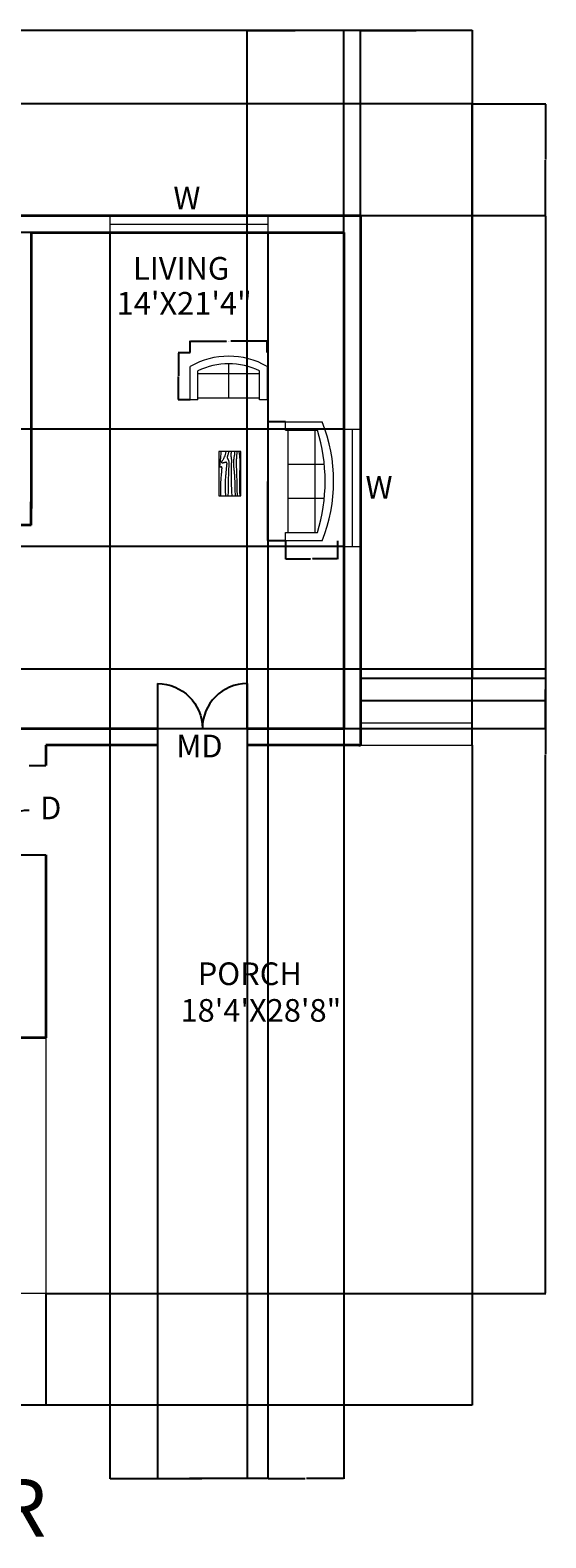
# Model space of a CAD drawing. Units: feet. Extents: x 2270 to 3094, y 1543 to 2352.
# Tile 6 of 6: x 2817 to 3094, y 1543 to 2352. Entities that reach past the tile are written whole.
import ezdxf

# ---------------------------------------------------------------- set-up
doc = ezdxf.new("R2010")
doc.units = ezdxf.units.FT
for name, color, linetype, lineweight in [('A-ANNO-DIMS', 2, 'Continuous', 18), ('A-ANNO-TEXT', 7, 'Continuous', 18), ('A-ANNO-TITL', 7, 'Continuous', 35), ('A-AREA-IDEN', 7, 'Continuous', 18), ('A-DOOR', 3, 'Continuous', 25), ('A-FLOR', 7, 'Continuous', 25), ('A-FLOR-STRS', 7, 'Continuous', 18), ('A-FURN', 8, 'Continuous', 18), ('A-GLAZ', 4, 'Continuous', 18), ('A-WALL', 7, 'Continuous', 35), ('C-PROP', 8, 'Continuous', 25)]:
    doc.layers.add(name, color=color, linetype=linetype, lineweight=lineweight)
doc.styles.get("Standard").update_dxf_attribs({"font": 'arial.ttf'})
doc.dimstyles.get("Standard").update_dxf_attribs({"dimtxt": 0.18, "dimasz": 0.18, "dimexe": 0.18, "dimexo": 0.0625, "dimgap": 0.09, "dimtad": 0, "dimtih": 1, "dimtoh": 1, "dimdec": 4, "dimzin": 0, "dimdsep": 46, "dimtxsty": 'Standard', "dimcen": 0.09, "dimadec": 0, "dimazin": 0, "dimtfac": 1, "dimtdec": 4, "dimtofl": 0, "dimtmove": 0, "dimatfit": 3, "dimfxl": 1, "dimtolj": 1, "dimtzin": 0, "dimarcsym": 0})

# ---------------------------------------------------------------- blocks, each defined once
blk = doc.blocks.new('Sofa - Roundback 7 ft.')
for p, q in [((-12.00002, -32.4421), (-12.00003, -6.5971)), ((11.99997, -32.4421), (11.99998, -6.5971)), ((-36.000027, -34), (-36.000027, -11.4696)), ((-35.999844, -13.3819), (35.9998, -13.3819)), ((35.99998, -34), (35.99998, -11.4696)), ((-36.000027, -32.4421), (35.99998, -32.4421))]:
    blk.add_line(p, q)
for points in [[(-36.000027, -34), (-42.000027, -34), (-42.000027, -8)], [(41.99998, -8), (41.99998, -34), (35.99998, -34)]]:
    blk.add_lwpolyline(points)
for centre, radius, start, end in [((0, -114.25), 114.25, 68.43141, 111.5686), ((-0.00001, -127.1968), 121.1968, 72.72033, 107.2797)]:
    blk.add_arc(centre, radius, start, end)
blk = doc.blocks.new('Sofa - Roundback Loveseat 5 ft.')
for p, q in [((-24, -33.99998), (-24, -11.46958)), ((0, -32.44198), (0, -5.99998)), ((24.00004, -33.99998), (24.00004, -11.46958)), ((-23.9998, -13.38178), (23.99986, -13.38178)), ((-24, -32.44198), (24.00004, -32.44198))]:
    blk.add_line(p, q)
for points in [[(-24, -33.99998), (-30, -33.99998), (-30, -7.99998)], [(30.00004, -7.99998), (30.00004, -33.99998), (24.00004, -33.99998)]]:
    blk.add_lwpolyline(points)
for centre, radius, start, end in [((0, -60.24998), 60.24998, 60.13715, 119.8628), ((0, -61.38438), 55.38444, 64.32083, 115.6792)]:
    blk.add_arc(centre, radius, start, end)
blk = doc.blocks.new('Table - Rectangular Woodgrain 60 x 30 in.')
for p, q in [((0, 0), (0, -30)), ((60, 0), (0, 0)), ((60, -30), (60, 0)), ((0, -30), (60, -30))]:
    blk.add_line(p, q)
for points in [[(0, -2.4), (4.8155, -2.418), (9.0302, -2.4688), (12.709, -2.5477), (15.9167, -2.65), (18.7181, -2.7711), (21.1781, -2.9063), (23.3616, -3.0508), (25.3333, -3.2), (27.1477, -3.3495), (28.8172, -3.4958), (30.3437, -3.636), (31.7291, -3.7667), (32.9756, -3.8849), (34.0849, -3.9875), (35.059, -4.0714), (35.9, -4.1334), (36.6114, -4.1711), (37.2041, -4.1854), (37.6906, -4.1779), (38.0833, -4.15), (38.3948, -4.1034), (38.6375, -4.0396), (38.8239, -3.9602), (38.9666, -3.8667), (39.0764, -3.7608), (39.1573, -3.6448), (39.2116, -3.521), (39.2416, -3.3917), (39.2498, -3.2593), (39.2385, -3.1261), (39.21, -2.9944), (39.1666, -2.8667), (39.111, -2.7447), (39.0468, -2.6281), (38.978, -2.5163), (38.9083, -2.4083), (38.8418, -2.3035), (38.7823, -2.201), (38.7337, -2.1001), (38.7, -2), (38.6844, -1.9003), (38.6875, -1.8021), (38.7094, -1.707), (38.75, -1.6167), (38.8094, -1.5326), (38.8875, -1.4563), (38.9844, -1.3893), (39.1, -1.3333), (39.2351, -1.2896), (39.3937, -1.2583), (39.5804, -1.2396), (39.8, -1.2333), (40.057, -1.2396), (40.3562, -1.2583), (40.7023, -1.2896), (41.1, -1.3333), (41.5547, -1.3895), (42.0755, -1.4573), (42.6721, -1.5361), (43.3542, -1.625), (44.1316, -1.7233), (45.014, -1.8302), (46.0114, -1.9449), (47.1333, -2.0667), (48.3862, -2.1947), (49.7625, -2.3281), (51.2513, -2.4663), (52.8416, -2.6083), (54.5226, -2.7535), (56.2833, -2.9011), (58.1127, -3.0501), (60, -3.2)], [(0, -9.2), (6.5759, -9.0858), (11.9385, -9.0365), (16.2527, -9.0418), (19.6833, -9.0917), (22.3952, -9.1759), (24.5531, -9.2844), (26.322, -9.4069), (27.8666, -9.5333), (29.3241, -9.6553), (30.7203, -9.7719), (32.0532, -9.8837), (33.3208, -9.9917), (34.5213, -10.0965), (35.6526, -10.199), (36.7128, -10.2999), (37.7, -10.4), (38.6129, -10.4996), (39.4531, -10.5969), (40.223, -10.6895), (40.925, -10.775), (41.5613, -10.8512), (42.1344, -10.9156), (42.6465, -10.966), (43.1, -11), (43.4976, -11.0158), (43.8437, -11.0136), (44.143, -10.9942), (44.4, -10.9583), (44.6195, -10.9069), (44.8062, -10.8406), (44.9648, -10.7603), (45.1, -10.6667), (45.2155, -10.5598), (45.3114, -10.4365), (45.3871, -10.2929), (45.4416, -10.125), (45.4743, -9.929), (45.4844, -9.7011), (45.4709, -9.4371), (45.4333, -9.1333), (45.3716, -8.7883), (45.2896, -8.4104), (45.1919, -8.0107), (45.0833, -7.6), (44.9685, -7.1893), (44.8521, -6.7896), (44.7388, -6.4117), (44.6333, -6.0667), (44.54, -5.7628), (44.4614, -5.4979), (44.4001, -5.2675), (44.3583, -5.0667), (44.3384, -4.8909), (44.3427, -4.7354), (44.3736, -4.5956), (44.4333, -4.4667), (44.5236, -4.3453), (44.6427, -4.2333), (44.7884, -4.1339), (44.9583, -4.05), (45.1501, -3.9849), (45.3614, -3.9417), (45.59, -3.9234), (45.8333, -3.9333), (46.0915, -3.9749), (46.3734, -4.0531), (46.6906, -4.1736), (47.0542, -4.3417), (47.4756, -4.5629), (47.9661, -4.8427), (48.5372, -5.1866), (49.2, -5.6), (49.9676, -6.0844), (50.8594, -6.625), (51.8965, -7.2031), (53.1, -7.8), (54.491, -8.3969), (56.0906, -8.975), (57.9199, -9.5156), (60, -10)], [(0, -12.8), (5.1847, -12.9322), (9.6213, -13.0323), (13.3963, -13.1059), (16.5958, -13.1583), (19.3063, -13.1952), (21.614, -13.2219), (23.6054, -13.2439), (25.3666, -13.2667), (26.9728, -13.2947), (28.4531, -13.3281), (29.8256, -13.3663), (31.1083, -13.4083), (32.3191, -13.4535), (33.476, -13.501), (34.597, -13.5501), (35.7, -13.6), (36.7984, -13.6497), (37.8875, -13.6979), (38.9578, -13.743), (40, -13.7833), (41.0047, -13.8174), (41.9625, -13.8438), (42.864, -13.8607), (43.7, -13.8667), (44.4631, -13.8604), (45.1552, -13.8417), (45.7801, -13.8104), (46.3416, -13.7667), (46.8439, -13.7104), (47.2906, -13.6417), (47.6858, -13.5604), (48.0333, -13.4667), (48.3375, -13.3608), (48.6042, -13.2448), (48.8396, -13.121), (49.05, -12.9917), (49.2417, -12.8593), (49.4208, -12.7261), (49.5937, -12.5944), (49.7667, -12.4667), (49.9452, -12.3451), (50.1323, -12.2313), (50.3303, -12.1268), (50.5416, -12.0333), (50.7686, -11.9524), (51.0135, -11.8854), (51.2788, -11.8341), (51.5666, -11.8), (51.8785, -11.7843), (52.2116, -11.7865), (52.562, -11.8059), (52.926, -11.8417), (53.2998, -11.8931), (53.6795, -11.9594), (54.0614, -12.0397), (54.4416, -12.1333), (54.8223, -12.2401), (55.2293, -12.3625), (55.6942, -12.5037), (56.2489, -12.6667), (56.9251, -12.8547), (57.7545, -13.0708), (58.7689, -13.3182), (60, -13.6)], [(0, -18), (5.124, -17.7273), (9.6609, -17.5057), (13.6705, -17.3303), (17.2125, -17.1958), (20.3467, -17.0973), (23.1328, -17.0297), (25.6307, -16.9878), (27.9, -16.9667), (29.9928, -16.9617), (31.9302, -16.9703), (33.7254, -16.9907), (35.3917, -17.0208), (36.9423, -17.0588), (38.3906, -17.1026), (39.7499, -17.1503), (41.0333, -17.2), (42.2519, -17.2496), (43.4073, -17.2969), (44.4986, -17.3395), (45.525, -17.375), (46.4858, -17.4012), (47.3802, -17.4156), (48.2074, -17.416), (48.9667, -17.4), (49.6583, -17.3662), (50.2872, -17.3167), (50.8595, -17.2547), (51.3812, -17.1833), (51.8584, -17.1057), (52.2971, -17.025), (52.7034, -16.9443), (53.0833, -16.8667), (53.443, -16.7951), (53.789, -16.7313), (54.128, -16.6768), (54.4666, -16.6334), (54.8115, -16.6024), (55.1693, -16.5854), (55.5465, -16.5841), (55.95, -16.6), (56.3828, -16.6337), (56.8346, -16.6823), (57.2915, -16.7418), (57.7396, -16.8084), (58.165, -16.878), (58.5539, -16.9469), (58.8924, -17.0111), (59.1666, -17.0667), (59.3679, -17.1107), (59.5078, -17.1438), (59.6032, -17.1675), (59.6708, -17.1833), (59.7275, -17.193), (59.7901, -17.1979), (59.8753, -17.1998), (60, -17.2)], [(0, -22.4), (8.0098, -22.2501), (14.4094, -22.1011), (19.4168, -21.9535), (23.25, -21.8083), (26.1269, -21.6663), (28.2656, -21.5281), (29.884, -21.3947), (31.2, -21.2667), (32.3967, -21.1448), (33.5172, -21.0292), (34.5697, -20.9198), (35.5625, -20.8167), (36.5037, -20.7198), (37.4015, -20.6292), (38.2642, -20.5448), (39.1, -20.4667), (39.9164, -20.3951), (40.7187, -20.3313), (41.5117, -20.2768), (42.3, -20.2333), (43.0883, -20.2024), (43.8812, -20.1854), (44.6836, -20.1841), (45.5, -20.2), (46.3328, -20.234), (47.1747, -20.2844), (48.0163, -20.3488), (48.8479, -20.425), (49.66, -20.5106), (50.4429, -20.6031), (51.1872, -20.7004), (51.8833, -20.8), (52.5246, -20.8999), (53.1166, -20.9995), (53.6681, -21.0983), (54.1875, -21.1958), (54.6834, -21.2919), (55.1646, -21.3859), (55.6394, -21.4777), (56.1167, -21.5667), (56.6028, -21.6515), (57.0961, -21.7266), (57.5929, -21.7852), (58.0896, -21.8208), (58.5823, -21.8268), (59.0674, -21.7964), (59.5412, -21.723), (60, -21.6)], [(0, -25.2), (8.6355, -25.0504), (15.7026, -24.9031), (21.4049, -24.7606), (25.9458, -24.625), (29.529, -24.4988), (32.3578, -24.3844), (34.6359, -24.284), (36.5667, -24.2), (38.3213, -24.1341), (39.9417, -24.0854), (41.437, -24.0523), (42.8167, -24.0333), (44.0901, -24.0268), (45.2667, -24.0313), (46.3557, -24.0451), (47.3667, -24.0667), (48.309, -24.0947), (49.1928, -24.1287), (50.0284, -24.168), (50.826, -24.2125), (51.5959, -24.2617), (52.3483, -24.3151), (53.0935, -24.3725), (53.8417, -24.4334), (54.6009, -24.497), (55.3699, -24.561), (56.1454, -24.6226), (56.9239, -24.6792), (57.7021, -24.7279), (58.4764, -24.7662), (59.2435, -24.7911), (60, -24.8)], [(0, -28.8), (5.6867, -28.6681), (10.45, -28.5698), (14.407, -28.5012), (17.675, -28.4584), (20.3711, -28.4374), (22.6125, -28.4344), (24.5164, -28.4455), (26.2, -28.4667), (27.762, -28.4947), (29.2276, -28.5281), (30.6033, -28.5663), (31.8958, -28.6084), (33.1118, -28.6535), (34.2578, -28.7011), (35.3405, -28.7501), (36.3666, -28.8), (37.3443, -28.8497), (38.288, -28.8974), (39.2137, -28.9412), (40.1375, -28.9792), (41.0753, -29.0093), (42.0432, -29.0297), (43.0572, -29.0384), (44.1333, -29.0333), (45.2936, -29.0114), (46.5843, -28.9641), (48.0579, -28.8816), (49.7666, -28.7542), (51.7629, -28.5721), (54.0989, -28.3255), (56.8272, -28.0048), (60, -27.6)]]:
    blk.add_lwpolyline(points)
blk = doc.blocks.new('DOOR-SWING-24')
blk.add_line((33, 0), (0, 0))
blk.add_arc((9, 0), 24, 0, 90)
blk = doc.blocks.new('*D18')
at = {"layer": 'A-ANNO-DIMS', "color": 0, "lineweight": -2, "transparency": 16777216}
for p, q in [((2954.26, 2141.51), (2944.57, 2141.51)), ((2944.75, 2141.33), (2944.75, 2109.77)), ((2944.75, 2077.85), (2944.75, 2109.41)), ((2954.26, 2077.67), (2944.57, 2077.67))]:
    blk.add_line(p, q, dxfattribs=at)
at = {"layer": 'A-ANNO-DIMS', "color": 0, "transparency": 16777216}
for points in [[(2944.72, 2141.33), (2944.78, 2141.33), (2944.75, 2141.51)], [(2944.72, 2077.85), (2944.78, 2077.85), (2944.75, 2077.67)]]:
    blk.add_solid(points, dxfattribs=at)
at = {"layer": 'Defpoints', "color": 0, "transparency": 16777216}
for p in [(2954.33, 2141.51), (2944.75, 2077.67), (2954.33, 2077.67)]:
    blk.add_point(p, dxfattribs=at)
at = {"layer": 'A-ANNO-DIMS', "color": 0, "transparency": 16777216, "insert": (2944.75, 2109.59), "char_height": 0.18, "attachment_point": 5}
blk.add_mtext('\\A1;SOFA 64 TYP.', dxfattribs=at)
blk = doc.blocks.new('*D19')
at = {"layer": 'A-ANNO-DIMS', "color": 0, "lineweight": -2, "transparency": 16777216}
for p, q in [((2954.33, 2077.6), (2954.33, 2067.91)), ((2982.2, 2077.6), (2982.2, 2067.91)), ((2954.51, 2068.09), (2967.73, 2068.09)), ((2982.02, 2068.09), (2968.79, 2068.09))]:
    blk.add_line(p, q, dxfattribs=at)
at = {"layer": 'A-ANNO-DIMS', "color": 0, "transparency": 16777216}
for points in [[(2954.51, 2068.12), (2954.51, 2068.06), (2954.33, 2068.09)], [(2982.02, 2068.12), (2982.02, 2068.06), (2982.2, 2068.09)]]:
    blk.add_solid(points, dxfattribs=at)
at = {"layer": 'Defpoints', "color": 0, "transparency": 16777216}
for p in [(2954.33, 2077.67), (2982.2, 2077.67), (2982.2, 2068.09)]:
    blk.add_point(p, dxfattribs=at)
at = {"layer": 'A-ANNO-DIMS', "color": 0, "transparency": 16777216, "insert": (2968.26, 2068.09), "char_height": 0.18, "attachment_point": 5}
blk.add_mtext('\\A1;28 TYP.', dxfattribs=at)
blk = doc.blocks.new('*D20')
at = {"layer": 'A-ANNO-DIMS', "color": 0, "lineweight": -2, "transparency": 16777216}
for p, q in [((2903.14, 2178.61), (2903.14, 2184.93)), ((2903.32, 2184.75), (2922.59, 2184.75)), ((2944.3, 2184.75), (2925.04, 2184.75)), ((2944.48, 2178.61), (2944.48, 2184.93))]:
    blk.add_line(p, q, dxfattribs=at)
at = {"layer": 'A-ANNO-DIMS', "color": 0, "transparency": 16777216}
for points in [[(2903.32, 2184.78), (2903.32, 2184.72), (2903.14, 2184.75)], [(2944.3, 2184.78), (2944.3, 2184.72), (2944.48, 2184.75)]]:
    blk.add_solid(points, dxfattribs=at)
at = {"layer": 'Defpoints', "color": 0, "transparency": 16777216}
for p in [(2944.48, 2184.75), (2903.14, 2178.55), (2944.48, 2178.55)]:
    blk.add_point(p, dxfattribs=at)
at = {"layer": 'A-ANNO-DIMS', "color": 0, "transparency": 16777216, "insert": (2923.81, 2184.75), "char_height": 0.18, "attachment_point": 5}
blk.add_mtext('\\A1;LOVESEAT 41 TYP.', dxfattribs=at)
blk = doc.blocks.new('*D21')
at = {"layer": 'A-ANNO-DIMS', "color": 0, "lineweight": -2, "transparency": 16777216}
for p, q in [((2903.08, 2178.55), (2896.76, 2178.55)), ((2896.94, 2178.37), (2896.94, 2166.1)), ((2896.94, 2153.46), (2896.94, 2165.73)), ((2903.08, 2153.28), (2896.76, 2153.28))]:
    blk.add_line(p, q, dxfattribs=at)
at = {"layer": 'A-ANNO-DIMS', "color": 0, "transparency": 16777216}
for points in [[(2896.91, 2178.37), (2896.97, 2178.37), (2896.94, 2178.55)], [(2896.91, 2153.46), (2896.97, 2153.46), (2896.94, 2153.28)]]:
    blk.add_solid(points, dxfattribs=at)
at = {"layer": 'Defpoints', "color": 0, "transparency": 16777216}
for p in [(2896.94, 2178.55), (2903.14, 2178.55), (2903.14, 2153.28)]:
    blk.add_point(p, dxfattribs=at)
at = {"layer": 'A-ANNO-DIMS', "color": 0, "transparency": 16777216, "insert": (2896.94, 2165.92), "char_height": 0.18, "attachment_point": 5}
blk.add_mtext('\\A1;25 TYP.', dxfattribs=at)
blk = doc.blocks.new('*D26')
at = {"layer": 'A-ANNO-DIMS', "color": 0, "lineweight": -2, "transparency": 16777216}
for p, q in [((2309.67, 2312.15), (2309.67, 2351.56)), ((2309.85, 2351.38), (2681.88, 2351.38)), ((3054.49, 2351.38), (2682.45, 2351.38)), ((3054.67, 2312.15), (3054.67, 2351.56))]:
    blk.add_line(p, q, dxfattribs=at)
at = {"layer": 'A-ANNO-DIMS', "color": 0, "transparency": 16777216}
for points in [[(2309.85, 2351.41), (2309.85, 2351.35), (2309.67, 2351.38)], [(3054.49, 2351.41), (3054.49, 2351.35), (3054.67, 2351.38)]]:
    blk.add_solid(points, dxfattribs=at)
at = {"layer": 'Defpoints', "color": 0, "transparency": 16777216}
for p in [(3054.67, 2351.38), (2309.67, 2312.08), (3054.67, 2312.08)]:
    blk.add_point(p, dxfattribs=at)
at = {"layer": 'A-ANNO-DIMS', "color": 0, "transparency": 16777216, "insert": (2682.17, 2351.38), "char_height": 0.18, "attachment_point": 5}
blk.add_mtext('\\A1;745', dxfattribs=at)
blk = doc.blocks.new('*D28')
at = {"layer": 'A-ANNO-DIMS', "color": 0, "lineweight": -2, "transparency": 16777216}
for p, q in [((2994.67, 2004.15), (2994.67, 2351.56)), ((2994.85, 2351.38), (3024.45, 2351.38)), ((3054.49, 2351.38), (3024.88, 2351.38)), ((3054.67, 2004.15), (3054.67, 2351.56))]:
    blk.add_line(p, q, dxfattribs=at)
at = {"layer": 'A-ANNO-DIMS', "color": 0, "transparency": 16777216}
for points in [[(2994.85, 2351.41), (2994.85, 2351.35), (2994.67, 2351.38)], [(3054.49, 2351.41), (3054.49, 2351.35), (3054.67, 2351.38)]]:
    blk.add_solid(points, dxfattribs=at)
at = {"layer": 'Defpoints', "color": 0, "transparency": 16777216}
for p in [(3054.67, 2351.38), (2994.67, 2004.08), (3054.67, 2004.08)]:
    blk.add_point(p, dxfattribs=at)
at = {"layer": 'A-ANNO-DIMS', "color": 0, "transparency": 16777216, "insert": (3024.67, 2351.38), "char_height": 0.18, "attachment_point": 5}
blk.add_mtext('\\A1;60', dxfattribs=at)
blk = doc.blocks.new('*D29')
at = {"layer": 'A-ANNO-DIMS', "color": 0, "lineweight": -2, "transparency": 16777216}
for p, q in [((3054.73, 2312.08), (3094.15, 2312.08)), ((3093.97, 2311.9), (3093.97, 2282.27)), ((3093.97, 2252.26), (3093.97, 2281.9)), ((2994.73, 2252.08), (3094.15, 2252.08))]:
    blk.add_line(p, q, dxfattribs=at)
at = {"layer": 'A-ANNO-DIMS', "color": 0, "transparency": 16777216}
for points in [[(3093.94, 2311.9), (3094, 2311.9), (3093.97, 2312.08)], [(3093.94, 2252.26), (3094, 2252.26), (3093.97, 2252.08)]]:
    blk.add_solid(points, dxfattribs=at)
at = {"layer": 'Defpoints', "color": 0, "transparency": 16777216}
for p in [(3054.67, 2312.08), (3093.97, 2312.08), (2994.67, 2252.08)]:
    blk.add_point(p, dxfattribs=at)
at = {"layer": 'A-ANNO-DIMS', "color": 0, "transparency": 16777216, "insert": (3093.97, 2282.08), "char_height": 0.18, "attachment_point": 5}
blk.add_mtext('\\A1;60', dxfattribs=at)
blk = doc.blocks.new('*D30')
at = {"layer": 'A-ANNO-DIMS', "color": 0, "lineweight": -2, "transparency": 16777216}
for p, q in [((2369.67, 2252.15), (2369.67, 2351.56)), ((2369.85, 2351.38), (2681.88, 2351.38)), ((2994.49, 2351.38), (2682.46, 2351.38)), ((2994.67, 2252.15), (2994.67, 2351.56))]:
    blk.add_line(p, q, dxfattribs=at)
at = {"layer": 'A-ANNO-DIMS', "color": 0, "transparency": 16777216}
for points in [[(2369.85, 2351.41), (2369.85, 2351.35), (2369.67, 2351.38)], [(2994.49, 2351.41), (2994.49, 2351.35), (2994.67, 2351.38)]]:
    blk.add_solid(points, dxfattribs=at)
at = {"layer": 'Defpoints', "color": 0, "transparency": 16777216}
for p in [(2994.67, 2351.38), (2369.67, 2252.08), (2994.67, 2252.08)]:
    blk.add_point(p, dxfattribs=at)
at = {"layer": 'A-ANNO-DIMS', "color": 0, "transparency": 16777216, "insert": (2682.17, 2351.38), "char_height": 0.18, "attachment_point": 5}
blk.add_mtext('\\A1;625', dxfattribs=at)
blk = doc.blocks.new('*D31')
at = {"layer": 'A-ANNO-DIMS', "color": 0, "lineweight": -2, "transparency": 16777216}
for p, q in [((2994.73, 2252.08), (3094.15, 2252.08)), ((3093.97, 2251.9), (3093.97, 1963.27)), ((3093.97, 1674.26), (3093.97, 1962.9)), ((2825.73, 1674.08), (3094.15, 1674.08))]:
    blk.add_line(p, q, dxfattribs=at)
at = {"layer": 'A-ANNO-DIMS', "color": 0, "transparency": 16777216}
for points in [[(3093.94, 2251.9), (3094, 2251.9), (3093.97, 2252.08)], [(3093.94, 1674.26), (3094, 1674.26), (3093.97, 1674.08)]]:
    blk.add_solid(points, dxfattribs=at)
at = {"layer": 'Defpoints', "color": 0, "transparency": 16777216}
for p in [(2994.67, 2252.08), (3093.97, 2252.08), (2825.67, 1674.08)]:
    blk.add_point(p, dxfattribs=at)
at = {"layer": 'A-ANNO-DIMS', "color": 0, "transparency": 16777216, "insert": (3093.97, 1963.08), "char_height": 0.18, "attachment_point": 5}
blk.add_mtext('\\A1;578', dxfattribs=at)
blk = doc.blocks.new('*D38')
at = {"layer": 'A-ANNO-DIMS', "color": 0, "lineweight": -2, "transparency": 16777216}
for p, q in [((2859.96, 2243.02), (2859.96, 1574.6)), ((2944.81, 2243.02), (2944.81, 1574.6)), ((2860.14, 1574.78), (2901.99, 1574.78)), ((2944.63, 1574.78), (2902.78, 1574.78))]:
    blk.add_line(p, q, dxfattribs=at)
at = {"layer": 'A-ANNO-DIMS', "color": 0, "transparency": 16777216}
for points in [[(2860.14, 1574.81), (2860.14, 1574.75), (2859.96, 1574.78)], [(2944.63, 1574.81), (2944.63, 1574.75), (2944.81, 1574.78)]]:
    blk.add_solid(points, dxfattribs=at)
at = {"layer": 'Defpoints', "color": 0, "transparency": 16777216}
for p in [(2859.96, 2243.08), (2944.81, 2243.08), (2944.81, 1574.78)]:
    blk.add_point(p, dxfattribs=at)
at = {"layer": 'A-ANNO-DIMS', "color": 0, "transparency": 16777216, "insert": (2902.39, 1574.78), "char_height": 0.18, "attachment_point": 5}
blk.add_mtext('\\A1;84.85', dxfattribs=at)
blk = doc.blocks.new('*D39')
at = {"layer": 'A-ANNO-DIMS', "color": 0, "lineweight": -2, "transparency": 16777216}
for p, q in [((2944.81, 2243.02), (2944.81, 1574.6)), ((2985.67, 2243.02), (2985.67, 1574.6)), ((2944.99, 1574.78), (2964.84, 1574.78)), ((2985.49, 1574.78), (2965.64, 1574.78))]:
    blk.add_line(p, q, dxfattribs=at)
at = {"layer": 'A-ANNO-DIMS', "color": 0, "transparency": 16777216}
for points in [[(2944.99, 1574.81), (2944.99, 1574.75), (2944.81, 1574.78)], [(2985.49, 1574.81), (2985.49, 1574.75), (2985.67, 1574.78)]]:
    blk.add_solid(points, dxfattribs=at)
at = {"layer": 'Defpoints', "color": 0, "transparency": 16777216}
for p in [(2944.81, 2243.08), (2985.67, 2243.08), (2985.67, 1574.78)]:
    blk.add_point(p, dxfattribs=at)
at = {"layer": 'A-ANNO-DIMS', "color": 0, "transparency": 16777216, "insert": (2965.24, 1574.78), "char_height": 0.18, "attachment_point": 5}
blk.add_mtext('\\A1;40.85', dxfattribs=at)
blk = doc.blocks.new('*D40')
at = {"layer": 'A-ANNO-DIMS', "color": 0, "lineweight": -2, "transparency": 16777216}
for p, q in [((2985.6, 2243.08), (2270.19, 2243.08)), ((2270.37, 2242.9), (2270.37, 2190.53)), ((2270.37, 2137.79), (2270.37, 2190.16)), ((2985.6, 2137.61), (2270.19, 2137.61))]:
    blk.add_line(p, q, dxfattribs=at)
at = {"layer": 'A-ANNO-DIMS', "color": 0, "transparency": 16777216}
for points in [[(2270.34, 2242.9), (2270.4, 2242.9), (2270.37, 2243.08)], [(2270.34, 2137.79), (2270.4, 2137.79), (2270.37, 2137.61)]]:
    blk.add_solid(points, dxfattribs=at)
at = {"layer": 'Defpoints', "color": 0, "transparency": 16777216}
for p in [(2985.67, 2243.08), (2270.37, 2137.61), (2985.67, 2137.61)]:
    blk.add_point(p, dxfattribs=at)
at = {"layer": 'A-ANNO-DIMS', "color": 0, "transparency": 16777216, "insert": (2270.37, 2190.35), "char_height": 0.18, "attachment_point": 5}
blk.add_mtext('\\A1;105.48', dxfattribs=at)
blk = doc.blocks.new('*D41')
at = {"layer": 'A-ANNO-DIMS', "color": 0, "lineweight": -2, "transparency": 16777216}
for p, q in [((2985.6, 2137.61), (2270.19, 2137.61)), ((2270.37, 2137.43), (2270.37, 2106.32)), ((2270.37, 2074.84), (2270.37, 2105.95)), ((2985.6, 2074.66), (2270.19, 2074.66))]:
    blk.add_line(p, q, dxfattribs=at)
at = {"layer": 'A-ANNO-DIMS', "color": 0, "transparency": 16777216}
for points in [[(2270.34, 2137.43), (2270.4, 2137.43), (2270.37, 2137.61)], [(2270.34, 2074.84), (2270.4, 2074.84), (2270.37, 2074.66)]]:
    blk.add_solid(points, dxfattribs=at)
at = {"layer": 'Defpoints', "color": 0, "transparency": 16777216}
for p in [(2985.67, 2137.61), (2270.37, 2074.66), (2985.67, 2074.66)]:
    blk.add_point(p, dxfattribs=at)
at = {"layer": 'A-ANNO-DIMS', "color": 0, "transparency": 16777216, "insert": (2270.37, 2106.14), "char_height": 0.18, "attachment_point": 5}
blk.add_mtext('\\A1;62.94', dxfattribs=at)
blk = doc.blocks.new('*D42')
at = {"layer": 'A-ANNO-DIMS', "color": 0, "lineweight": -2, "transparency": 16777216}
for p, q in [((2933.67, 1977.15), (2933.67, 2351.56)), ((2933.85, 2351.38), (2959.45, 2351.38)), ((2985.49, 2351.38), (2959.88, 2351.38)), ((2985.67, 1977.15), (2985.67, 2351.56))]:
    blk.add_line(p, q, dxfattribs=at)
at = {"layer": 'A-ANNO-DIMS', "color": 0, "transparency": 16777216}
for points in [[(2933.85, 2351.41), (2933.85, 2351.35), (2933.67, 2351.38)], [(2985.49, 2351.41), (2985.49, 2351.35), (2985.67, 2351.38)]]:
    blk.add_solid(points, dxfattribs=at)
at = {"layer": 'Defpoints', "color": 0, "transparency": 16777216}
for p in [(2985.67, 2351.38), (2933.67, 1977.08), (2985.67, 1977.08)]:
    blk.add_point(p, dxfattribs=at)
at = {"layer": 'A-ANNO-DIMS', "color": 0, "transparency": 16777216, "insert": (2959.67, 2351.38), "char_height": 0.18, "attachment_point": 5}
blk.add_mtext('\\A1;52', dxfattribs=at)
blk = doc.blocks.new('*D43')
at = {"layer": 'A-ANNO-DIMS', "color": 0, "lineweight": -2, "transparency": 16777216}
for p, q in [((2885.67, 1968.02), (2885.67, 1574.6)), ((2933.67, 1968.02), (2933.67, 1574.6)), ((2885.85, 1574.78), (2909.44, 1574.78)), ((2933.49, 1574.78), (2909.89, 1574.78))]:
    blk.add_line(p, q, dxfattribs=at)
at = {"layer": 'A-ANNO-DIMS', "color": 0, "transparency": 16777216}
for points in [[(2885.85, 1574.81), (2885.85, 1574.75), (2885.67, 1574.78)], [(2933.49, 1574.81), (2933.49, 1574.75), (2933.67, 1574.78)]]:
    blk.add_solid(points, dxfattribs=at)
at = {"layer": 'Defpoints', "color": 0, "transparency": 16777216}
for p in [(2885.67, 1968.08), (2933.67, 1968.08), (2933.67, 1574.78)]:
    blk.add_point(p, dxfattribs=at)
at = {"layer": 'A-ANNO-DIMS', "color": 0, "transparency": 16777216, "insert": (2909.67, 1574.78), "char_height": 0.18, "attachment_point": 5}
blk.add_mtext('\\A1;48', dxfattribs=at)
blk = doc.blocks.new('*D56')
at = {"layer": 'A-ANNO-DIMS', "color": 0, "lineweight": -2, "transparency": 16777216}
for p, q in [((2378.73, 2009.08), (3094.15, 2009.08)), ((3093.97, 2008.9), (3093.97, 1993.27)), ((3093.97, 1977.26), (3093.97, 1992.9)), ((2378.73, 1977.08), (3094.15, 1977.08))]:
    blk.add_line(p, q, dxfattribs=at)
at = {"layer": 'A-ANNO-DIMS', "color": 0, "transparency": 16777216}
for points in [[(3093.94, 2008.9), (3094, 2008.9), (3093.97, 2009.08)], [(3093.94, 1977.26), (3094, 1977.26), (3093.97, 1977.08)]]:
    blk.add_solid(points, dxfattribs=at)
at = {"layer": 'Defpoints', "color": 0, "transparency": 16777216}
for p in [(2378.67, 2009.08), (3093.97, 2009.08), (2378.67, 1977.08)]:
    blk.add_point(p, dxfattribs=at)
at = {"layer": 'A-ANNO-DIMS', "color": 0, "transparency": 16777216, "insert": (3093.97, 1993.08), "char_height": 0.18, "attachment_point": 5}
blk.add_mtext('\\A1;32', dxfattribs=at)
blk = doc.blocks.new('*D68')
at = {"layer": 'A-ANNO-DIMS', "color": 0, "lineweight": -2, "transparency": 16777216}
for p, q in [((2994.73, 2004.08), (3094.15, 2004.08)), ((3093.97, 2003.9), (3093.97, 1998.26)), ((3093.97, 1992.26), (3093.97, 1997.9)), ((2994.73, 1992.08), (3094.15, 1992.08))]:
    blk.add_line(p, q, dxfattribs=at)
at = {"layer": 'A-ANNO-DIMS', "color": 0, "transparency": 16777216}
for points in [[(3093.94, 2003.9), (3094, 2003.9), (3093.97, 2004.08)], [(3093.94, 1992.26), (3094, 1992.26), (3093.97, 1992.08)]]:
    blk.add_solid(points, dxfattribs=at)
at = {"layer": 'Defpoints', "color": 0, "transparency": 16777216}
for p in [(2994.67, 2004.08), (2994.67, 1992.08), (3093.97, 1992.08)]:
    blk.add_point(p, dxfattribs=at)
at = {"layer": 'A-ANNO-DIMS', "color": 0, "transparency": 16777216, "insert": (3093.97, 1998.08), "char_height": 0.18, "attachment_point": 5}
blk.add_mtext('\\A1;12', dxfattribs=at)

msp = doc.modelspace()

# ---------------------------------------------------------------- linework, layer by layer
at = {"layer": 'A-DOOR'}
msp.add_line((2816.6659, 1957.2599), (2825.6659, 1957.2599), dxfattribs=at)
at = {"layer": 'A-FLOR'}
msp.add_line((2825.6659, 1674.0845), (2825.6659, 1614.0845), dxfattribs=at)
at = {"layer": 'A-FLOR-STRS'}
for p, q in [((2994.6659, 2004.0845), (3054.6659, 2004.0845)), ((2994.6659, 1992.0845), (3054.6659, 1992.0845)), ((2994.6659, 1980.0845), (3054.6659, 1980.0845)), ((2994.6659, 1968.0845), (3054.6659, 1968.0845))]:
    msp.add_line(p, q, dxfattribs=at)
msp.add_lwpolyline([(2825.6659, 1811.0845), (2825.6659, 1674.0845), (2664.6659, 1674.0845)], dxfattribs=at)
at = {"layer": 'A-GLAZ'}
for p, q in [((2859.9591, 2252.0845), (2859.9591, 2243.0845)), ((2944.8128, 2252.0845), (2944.8128, 2243.0845)), ((2859.9591, 2247.5845), (2944.8128, 2247.5845)), ((2985.6659, 2137.6089), (2994.6659, 2137.6089)), ((2990.1659, 2137.6089), (2990.1659, 2074.664)), ((2985.6659, 2074.664), (2994.6659, 2074.664))]:
    msp.add_line(p, q, dxfattribs=at)
at = {"layer": 'A-WALL'}
for p, q in [((2369.6659, 2252.0845), (2994.6659, 2252.0845)), ((2994.6659, 2252.0845), (2994.6659, 1968.0845)), ((2817.6659, 2243.0845), (2817.6659, 2095.0845)), ((2817.6659, 2243.0845), (2985.6659, 2243.0845)), ((2985.6659, 2243.0845), (2985.6659, 1977.0845)), ((2817.6659, 2086.0845), (2817.6659, 2098.6012)), ((2817.6659, 2086.0845), (2679.6659, 2086.0845)), ((2803.9581, 1977.0845), (2885.6659, 1977.0845)), ((2933.6659, 1977.0845), (2985.6659, 1977.0845)), ((2825.6659, 1968.0845), (2825.6659, 1957.2599)), ((2885.6659, 1968.0845), (2825.6659, 1968.0845)), ((2993.6659, 1968.0845), (2933.6659, 1968.0845)), ((2993.6659, 1968.0845), (2994.6659, 1968.0845)), ((2825.6659, 1909.2599), (2825.6659, 1811.0845)), ((2825.6659, 1811.0845), (2664.6659, 1811.0845))]:
    msp.add_line(p, q, dxfattribs=at)
at = {"layer": 'C-PROP'}
for p, q in [((3054.6659, 2312.0845), (2369.6659, 2312.0845)), ((3054.6659, 2252.0845), (3054.6659, 2312.0845)), ((3054.6659, 1968.0845), (3054.6659, 2252.0845)), ((3054.6659, 1968.0845), (3054.6659, 1614.0845)), ((3054.6659, 1614.0845), (2309.6659, 1614.0845))]:
    msp.add_line(p, q, dxfattribs=at)

# ---------------------------------------------------------------- block references
at = {"layer": 'A-DOOR', "extrusion": (0, 0, -1), "zscale": -1, "rotation": 90.00000000000003}
msp.add_blockref('DOOR-SWING-24', (-2885.6664, 1968.0846), dxfattribs=at)
at = {"layer": 'A-DOOR', "rotation": 89.99999999999955}
msp.add_blockref('DOOR-SWING-24', (2933.6654, 1968.0846), dxfattribs=at)
at = {"layer": 'A-DOOR', "extrusion": (0, 0, -1), "zscale": -1}
msp.add_blockref('DOOR-SWING-24', (-2825.6658, 1909.2604), dxfattribs=at)
at = {"layer": 'A-FURN', "xscale": 0.6890107561229493, "yscale": 0.6890107561229493, "zscale": 0.6890107561229493}
msp.add_blockref('Sofa - Roundback Loveseat 5 ft.', (2923.8145, 2176.7103), dxfattribs=at)
at = {"layer": 'A-FURN'}
for name, p, xscale, yscale, zscale, rotation in [('Sofa - Roundback 7 ft.', (2980.1688, 2109.5904), 0.7600860967180219, 0.7600860967180219, 0.7600860967180219, 269.9999778310005), ('Table - Rectangular Woodgrain 60 x 30 in.', (2918.578, 2101.8863), 0.3935928378760143, 0.3935928378760143, 0.3935928378760143, 90)]:
    msp.add_blockref(name, p, dxfattribs=dict(at, xscale=xscale, yscale=yscale, zscale=zscale, rotation=rotation))

# ---------------------------------------------------------------- texts
at = {"layer": 'A-ANNO-TEXT'}
for s, height, p in [('W', 12.1456, (2894.0898, 2255.5534)), ('W', 12.1456, (2997.2706, 2100.3452)), ('MD', 12.14556, (2895.6836, 1961.5453)), ('D', 12.1456, (2822.555, 1928.3414))]:
    msp.add_text(s, height=height, dxfattribs=at).set_placement(p)
at = {"layer": 'A-ANNO-TITL'}
msp.add_text('GROUND FLOOR', height=31.058177, dxfattribs=at).set_placement((2502.4393, 1543.4965))
at = {"layer": 'A-AREA-IDEN'}
for s, height, p in [('LIVING', 12.14556, (2872.442, 2217.7462)), ('14\'X21\'4"', 12.14556, (2863.6322, 2199.0009)), ('PORCH', 12.14556, (2907.1838, 1839.4164)), ('18\'4\'X28\'8"', 12.145557, (2897.9295, 1819.7561))]:
    msp.add_text(s, height=height, dxfattribs=at).set_placement(p)

# ---------------------------------------------------------------- dimensions: what is measured, and where the dimension line sits
at = {"layer": 'A-ANNO-DIMS'}
for base, p1, p2, override, picture, middle in [((3054.6659, 2351.3845), (2309.6659, 2312.0845), (3054.6659, 2312.0845), {"dimdec": 0, "dimlfac": 1, "dimrnd": 0, "dimzin": 0, "dimdsep": 46, "dimlunit": 2}, '*D26', (2682.1659, 2351.3845)), ((2994.6659, 2351.3845), (2369.6659, 2252.0845), (2994.6659, 2252.0845), {"dimdec": 0, "dimlfac": 1, "dimrnd": 0, "dimzin": 0, "dimdsep": 46, "dimlunit": 2}, '*D30', (2682.1659, 2351.3845)), ((2985.6659, 2351.3845), (2933.6659, 1977.0845), (2985.6659, 1977.0845), {"dimdec": 0, "dimlfac": 1, "dimrnd": 0, "dimzin": 0, "dimdsep": 46, "dimlunit": 2}, '*D42', (2959.6659, 2351.3845)), ((3054.6659, 2351.3845), (2994.6659, 2004.0845), (3054.6659, 2004.0845), {"dimdec": 0, "dimlfac": 1, "dimrnd": 0, "dimzin": 0, "dimdsep": 46, "dimlunit": 2}, '*D28', (3024.6659, 2351.3845)), ((2944.8128, 1574.7845), (2859.9591, 2243.0845), (2944.8128, 2243.0845), {"dimdec": 2, "dimlfac": 1, "dimrnd": 0, "dimzin": 0, "dimdsep": 46, "dimlunit": 2}, '*D38', (2902.3859, 1574.7845)), ((2985.6659, 1574.7845), (2944.8128, 2243.0845), (2985.6659, 2243.0845), {"dimdec": 2, "dimlfac": 1, "dimrnd": 0, "dimzin": 0, "dimdsep": 46, "dimlunit": 2}, '*D39', (2965.2393, 1574.7845)), ((2933.6659, 1574.7845), (2885.6659, 1968.0845), (2933.6659, 1968.0845), {"dimdec": 0, "dimlfac": 1, "dimrnd": 0, "dimzin": 0, "dimdsep": 46, "dimlunit": 2}, '*D43', (2909.6659, 1574.7845))]:
    dim = msp.add_linear_dim(base=base, p1=p1, p2=p2, dimstyle='Standard', override=override, dxfattribs=at)
    dim.commit()
    dim.dimension.update_dxf_attribs({"geometry": picture, "text_midpoint": middle})
for base, p1, p2, override, picture, middle in [((3093.9659, 2312.0845), (2994.6659, 2252.0845), (3054.6659, 2312.0845), {"dimdec": 0, "dimlfac": 1, "dimrnd": 0, "dimzin": 0, "dimdsep": 46, "dimlunit": 2}, '*D29', (3093.9659, 2282.0845)), ((3093.9659, 2252.0845), (2825.6659, 1674.0845), (2994.6659, 2252.0845), {"dimdec": 0, "dimlfac": 1, "dimrnd": 0, "dimzin": 0, "dimdsep": 46, "dimlunit": 2}, '*D31', (3093.9659, 1963.0845)), ((2270.3659, 2137.6089), (2985.6659, 2243.0845), (2985.6659, 2137.6089), {"dimdec": 2, "dimlfac": 1, "dimrnd": 0, "dimzin": 0, "dimdsep": 46, "dimlunit": 2}, '*D40', (2270.3659, 2190.3467)), ((2270.3659, 2074.664), (2985.6659, 2137.6089), (2985.6659, 2074.664), {"dimdec": 2, "dimlfac": 1, "dimrnd": 0, "dimzin": 0, "dimdsep": 46, "dimlunit": 2}, '*D41', (2270.3659, 2106.1365)), ((3093.9659, 2009.0845), (2378.6659, 1977.0845), (2378.6659, 2009.0845), {"dimdec": 0, "dimlfac": 1, "dimrnd": 0, "dimzin": 0, "dimdsep": 46, "dimlunit": 2}, '*D56', (3093.9659, 1993.0845)), ((3093.9659, 1992.0845), (2994.6659, 2004.0845), (2994.6659, 1992.0845), {"dimdec": 0, "dimlfac": 1, "dimrnd": 0, "dimzin": 0, "dimdsep": 46, "dimlunit": 2}, '*D68', (3093.9659, 1998.0845))]:
    dim = msp.add_linear_dim(base=base, p1=p1, p2=p2, angle=90, dimstyle='Standard', override=override, dxfattribs=at)
    dim.commit()
    dim.dimension.update_dxf_attribs({"geometry": picture, "text_midpoint": middle})
dim = msp.add_linear_dim(base=(2944.4849, 2184.7488), p1=(2903.1442, 2178.5477), p2=(2944.4849, 2178.5477), text='LOVESEAT <> TYP.', dimstyle='Standard', override={"dimdec": 0, "dimlfac": 1, "dimrnd": 0, "dimzin": 0, "dimdsep": 46, "dimlunit": 2}, dxfattribs=at)
dim.commit()
dim.dimension.update_dxf_attribs({"geometry": '*D20', "text_midpoint": (2923.8145, 2184.7488)})
for base, p1, p2, angle, text, picture, middle in [((2896.9431, 2178.5477), (2903.1442, 2153.2839), (2903.1442, 2178.5477), 90, '<> TYP.', '*D21', (2896.9431, 2165.9158)), ((2944.7488, 2077.6668), (2954.3259, 2141.514), (2954.3258, 2077.6668), 269.9999778, 'SOFA <> TYP.', '*D18', (2944.7488, 2109.5904)), ((2982.1957, 2068.0897), (2954.3258, 2077.6668), (2982.1957, 2077.6668), 359.9999778, '<> TYP.', '*D19', (2968.2607, 2068.0897))]:
    dim = msp.add_linear_dim(base=base, p1=p1, p2=p2, angle=angle, text=text, dimstyle='Standard', override={"dimdec": 0, "dimlfac": 1, "dimrnd": 0, "dimzin": 0, "dimdsep": 46, "dimlunit": 2}, dxfattribs=at)
    dim.commit()
    dim.dimension.update_dxf_attribs({"geometry": picture, "text_midpoint": middle})

doc.saveas('drawing.dxf')
